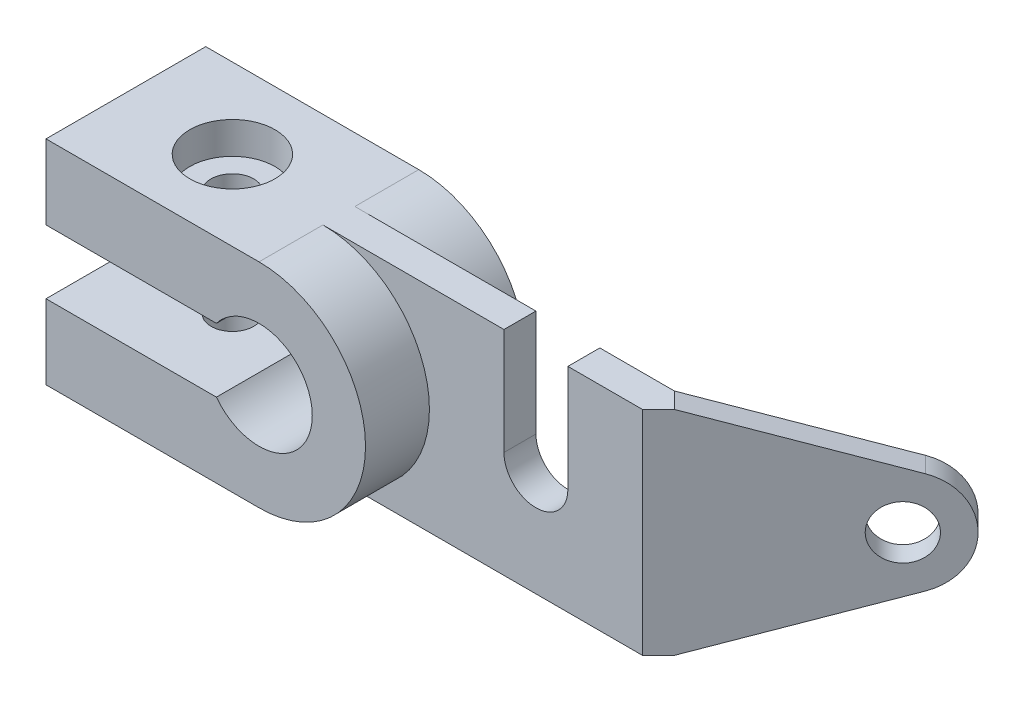
ISO-10303-21;
HEADER;
FILE_DESCRIPTION(('STEP AP214'),'2;1');
FILE_NAME('part.step','',(''),(''),'','','');
FILE_SCHEMA(('AUTOMOTIVE_DESIGN { 1 0 10303 214 1 1 1 1 }'));
ENDSEC;
DATA;
#1=APPLICATION_CONTEXT('core data for automotive mechanical design processes');
#2=APPLICATION_PROTOCOL_DEFINITION('international standard','automotive_design',2000,#1);
#3=PRODUCT_CONTEXT('',#1,'mechanical');
#4=PRODUCT('Part','Part','',(#3));
#5=PRODUCT_RELATED_PRODUCT_CATEGORY('part','',(#4));
#6=PRODUCT_DEFINITION_FORMATION('','',#4);
#7=PRODUCT_DEFINITION_CONTEXT('part definition',#1,'design');
#8=PRODUCT_DEFINITION('design','',#6,#7);
#9=PRODUCT_DEFINITION_SHAPE('','',#8);
#10=(LENGTH_UNIT() NAMED_UNIT(*) SI_UNIT(.MILLI.,.METRE.));
#11=(NAMED_UNIT(*) PLANE_ANGLE_UNIT() SI_UNIT($,.RADIAN.));
#12=(NAMED_UNIT(*) SI_UNIT($,.STERADIAN.) SOLID_ANGLE_UNIT());
#13=UNCERTAINTY_MEASURE_WITH_UNIT(LENGTH_MEASURE(1.E-05),#10,'distance_accuracy_value','');
#14=(GEOMETRIC_REPRESENTATION_CONTEXT(3) GLOBAL_UNCERTAINTY_ASSIGNED_CONTEXT((#13)) GLOBAL_UNIT_ASSIGNED_CONTEXT((#10,
#11,#12)) REPRESENTATION_CONTEXT('',''));
#15=CARTESIAN_POINT('',(0.,0.,0.));
#16=DIRECTION('',(0.,0.,1.));
#17=DIRECTION('',(1.,0.,0.));
#18=AXIS2_PLACEMENT_3D('',#15,#16,#17);
#19=CARTESIAN_POINT('',(90.,30.,4.5));
#20=DIRECTION('',(-0.707106781186549,0.,-0.707106781186546));
#21=DIRECTION('',(-0.707106781186546,0.,0.707106781186549));
#22=AXIS2_PLACEMENT_3D('',#19,#20,#21);
#23=PLANE('',#22);
#24=CARTESIAN_POINT('',(126.673358543988,0.,-32.173358543988));
#25=DIRECTION('',(-0.707106781186549,0.,-0.707106781186546));
#26=DIRECTION('',(-0.707106781186546,0.,0.707106781186549));
#27=AXIS2_PLACEMENT_3D('',#24,#25,#26);
#28=CIRCLE('',#27,7.50000000000002);
#29=CARTESIAN_POINT('',(121.370057685089,0.,-26.8700576850888));
#30=VERTEX_POINT('',#29);
#31=EDGE_CURVE('E220',#30,#30,#28,.T.);
#32=ORIENTED_EDGE('',*,*,#31,.T.);
#33=EDGE_LOOP('',(#32));
#34=FACE_BOUND('',#33,.T.);
#35=DIRECTION('',(0.674665588129938,0.299420587780075,-0.674665588129941));
#36=VECTOR('',#35,1.);
#37=CARTESIAN_POINT('',(102.523963114911,-26.4389175993817,-8.02396311491096));
#38=LINE('',#37,#36);
#39=CARTESIAN_POINT('',(94.5,-30.,0.));
#40=VERTEX_POINT('',#39);
#41=CARTESIAN_POINT('',(129.84919346468,-14.3118183719967,-35.3491934646803));
#42=VERTEX_POINT('',#41);
#43=EDGE_CURVE('E197',#40,#42,#38,.T.);
#44=ORIENTED_EDGE('',*,*,#43,.T.);
#45=CARTESIAN_POINT('',(126.673358543988,0.,-32.173358543988));
#46=DIRECTION('',(-0.707106781186549,0.,-0.707106781186546));
#47=DIRECTION('',(-0.707106781186546,0.,0.707106781186549));
#48=AXIS2_PLACEMENT_3D('',#45,#46,#47);
#49=CIRCLE('',#48,15.);
#50=CARTESIAN_POINT('',(129.84919346468,14.3118183719967,-35.3491934646803));
#51=VERTEX_POINT('',#50);
#52=EDGE_CURVE('E358',#51,#42,#49,.T.);
#53=ORIENTED_EDGE('',*,*,#52,.F.);
#54=DIRECTION('',(-0.674665588129938,0.299420587780076,0.674665588129941));
#55=VECTOR('',#54,1.);
#56=CARTESIAN_POINT('',(90.4034370977395,31.8180789025757,4.09656290226045));
#57=LINE('',#56,#55);
#58=CARTESIAN_POINT('',(94.5,30.,0.));
#59=VERTEX_POINT('',#58);
#60=EDGE_CURVE('E352',#51,#59,#57,.T.);
#61=ORIENTED_EDGE('',*,*,#60,.T.);
#62=DIRECTION('',(0.707106781186546,0.,-0.707106781186549));
#63=VECTOR('',#62,1.);
#64=CARTESIAN_POINT('',(90.,30.,4.5));
#65=LINE('',#64,#63);
#66=CARTESIAN_POINT('',(90.,30.,4.5));
#67=VERTEX_POINT('',#66);
#68=EDGE_CURVE('E353',#67,#59,#65,.T.);
#69=ORIENTED_EDGE('',*,*,#68,.F.);
#70=DIRECTION('',(0.,-1.,0.));
#71=VECTOR('',#70,1.);
#72=CARTESIAN_POINT('',(90.,30.,4.5));
#73=LINE('',#72,#71);
#74=CARTESIAN_POINT('',(90.,-30.,4.5));
#75=VERTEX_POINT('',#74);
#76=EDGE_CURVE('E222',#67,#75,#73,.T.);
#77=ORIENTED_EDGE('',*,*,#76,.T.);
#78=DIRECTION('',(0.707106781186546,0.,-0.707106781186549));
#79=VECTOR('',#78,1.);
#80=CARTESIAN_POINT('',(90.,-30.,4.5));
#81=LINE('',#80,#79);
#82=EDGE_CURVE('E218',#75,#40,#81,.T.);
#83=ORIENTED_EDGE('',*,*,#82,.T.);
#84=EDGE_LOOP('',(#44,#53,#61,#69,#77,#83));
#85=FACE_BOUND('',#84,.T.);
#86=ADVANCED_FACE('F69',(#34,#85),#23,.F.);
#87=CARTESIAN_POINT('',(132.779960261786,30.,-47.2799602617859));
#88=DIRECTION('',(0.707106781186544,0.,0.707106781186551));
#89=DIRECTION('',(0.707106781186551,0.,-0.707106781186544));
#90=AXIS2_PLACEMENT_3D('',#87,#88,#89);
#91=PLANE('',#90);
#92=CARTESIAN_POINT('',(122.173358543988,0.,-36.6733585439877));
#93=DIRECTION('',(0.707106781186544,0.,0.707106781186551));
#94=DIRECTION('',(0.707106781186551,0.,-0.707106781186544));
#95=AXIS2_PLACEMENT_3D('',#92,#93,#94);
#96=CIRCLE('',#95,7.50000000000002);
#97=CARTESIAN_POINT('',(127.476659402887,0.,-41.9766594028868));
#98=VERTEX_POINT('',#97);
#99=EDGE_CURVE('E71',#98,#98,#96,.T.);
#100=ORIENTED_EDGE('',*,*,#99,.T.);
#101=EDGE_LOOP('',(#100));
#102=FACE_BOUND('',#101,.T.);
#103=CARTESIAN_POINT('',(122.173358543988,0.,-36.6733585439877));
#104=DIRECTION('',(0.707106781186544,0.,0.707106781186551));
#105=DIRECTION('',(0.707106781186551,0.,-0.707106781186544));
#106=AXIS2_PLACEMENT_3D('',#103,#104,#105);
#107=CIRCLE('',#106,15.);
#108=CARTESIAN_POINT('',(125.34919346468,-14.3118183719967,-39.84919346468));
#109=VERTEX_POINT('',#108);
#110=CARTESIAN_POINT('',(125.34919346468,14.3118183719967,-39.84919346468));
#111=VERTEX_POINT('',#110);
#112=EDGE_CURVE('E12',#109,#111,#107,.T.);
#113=ORIENTED_EDGE('',*,*,#112,.F.);
#114=DIRECTION('',(-0.674665588129943,-0.299420587780075,0.674665588129936));
#115=VECTOR('',#114,1.);
#116=CARTESIAN_POINT('',(141.065147832418,-7.33698465125482,-55.5651478324177));
#117=LINE('',#116,#115);
#118=CARTESIAN_POINT('',(90.,-30.,-4.5));
#119=VERTEX_POINT('',#118);
#120=EDGE_CURVE('E209',#109,#119,#117,.T.);
#121=ORIENTED_EDGE('',*,*,#120,.T.);
#122=DIRECTION('',(0.,-1.,0.));
#123=VECTOR('',#122,1.);
#124=CARTESIAN_POINT('',(90.,30.,-4.5));
#125=LINE('',#124,#123);
#126=CARTESIAN_POINT('',(90.,30.,-4.5));
#127=VERTEX_POINT('',#126);
#128=EDGE_CURVE('E231',#127,#119,#125,.T.);
#129=ORIENTED_EDGE('',*,*,#128,.F.);
#130=DIRECTION('',(0.674665588129943,-0.299420587780076,-0.674665588129936));
#131=VECTOR('',#130,1.);
#132=CARTESIAN_POINT('',(128.944621815247,12.7161459544488,-43.4446218152463));
#133=LINE('',#132,#131);
#134=EDGE_CURVE('E77',#127,#111,#133,.T.);
#135=ORIENTED_EDGE('',*,*,#134,.T.);
#136=EDGE_LOOP('',(#113,#121,#129,#135));
#137=FACE_BOUND('',#136,.T.);
#138=ADVANCED_FACE('F345',(#102,#137),#91,.F.);
#139=CARTESIAN_POINT('',(0.,30.,22.5));
#140=DIRECTION('',(0.,-1.,0.));
#141=DIRECTION('',(1.,0.,0.));
#142=AXIS2_PLACEMENT_3D('',#139,#140,#141);
#143=PLANE('',#142);
#144=CARTESIAN_POINT('',(-30.,30.,0.));
#145=DIRECTION('',(0.,1.,0.));
#146=DIRECTION('',(-1.,0.,0.));
#147=AXIS2_PLACEMENT_3D('',#144,#145,#146);
#148=CIRCLE('',#147,12.);
#149=CARTESIAN_POINT('',(-42.,30.,0.));
#150=VERTEX_POINT('',#149);
#151=EDGE_CURVE('E263',#150,#150,#148,.T.);
#152=ORIENTED_EDGE('',*,*,#151,.F.);
#153=EDGE_LOOP('',(#152));
#154=FACE_BOUND('',#153,.T.);
#155=DIRECTION('',(0.,0.,-1.));
#156=VECTOR('',#155,1.);
#157=CARTESIAN_POINT('',(51.,30.,25.5));
#158=LINE('',#157,#156);
#159=CARTESIAN_POINT('',(51.,30.,4.5));
#160=VERTEX_POINT('',#159);
#161=CARTESIAN_POINT('',(51.,30.,-4.5));
#162=VERTEX_POINT('',#161);
#163=EDGE_CURVE('E362',#160,#162,#158,.T.);
#164=ORIENTED_EDGE('',*,*,#163,.T.);
#165=DIRECTION('',(-1.,0.,0.));
#166=VECTOR('',#165,1.);
#167=CARTESIAN_POINT('',(0.,30.,-4.5));
#168=LINE('',#167,#166);
#169=CARTESIAN_POINT('',(0.,30.,-4.49999999999999));
#170=VERTEX_POINT('',#169);
#171=EDGE_CURVE('E382',#162,#170,#168,.T.);
#172=ORIENTED_EDGE('',*,*,#171,.T.);
#173=DIRECTION('',(0.,0.,-1.));
#174=VECTOR('',#173,1.);
#175=CARTESIAN_POINT('',(0.,30.,22.5));
#176=LINE('',#175,#174);
#177=CARTESIAN_POINT('',(0.,30.,-22.5));
#178=VERTEX_POINT('',#177);
#179=EDGE_CURVE('E316',#170,#178,#176,.T.);
#180=ORIENTED_EDGE('',*,*,#179,.T.);
#181=DIRECTION('',(-1.,0.,0.));
#182=VECTOR('',#181,1.);
#183=CARTESIAN_POINT('',(0.,30.,-22.5));
#184=LINE('',#183,#182);
#185=CARTESIAN_POINT('',(-60.,30.,-22.5));
#186=VERTEX_POINT('',#185);
#187=EDGE_CURVE('E293',#178,#186,#184,.T.);
#188=ORIENTED_EDGE('',*,*,#187,.T.);
#189=DIRECTION('',(0.,0.,-1.));
#190=VECTOR('',#189,1.);
#191=CARTESIAN_POINT('',(-60.,30.,22.5));
#192=LINE('',#191,#190);
#193=CARTESIAN_POINT('',(-60.,30.,22.5));
#194=VERTEX_POINT('',#193);
#195=EDGE_CURVE('E320',#194,#186,#192,.T.);
#196=ORIENTED_EDGE('',*,*,#195,.F.);
#197=DIRECTION('',(-1.,0.,0.));
#198=VECTOR('',#197,1.);
#199=CARTESIAN_POINT('',(0.,30.,22.5));
#200=LINE('',#199,#198);
#201=CARTESIAN_POINT('',(0.,30.,22.5));
#202=VERTEX_POINT('',#201);
#203=EDGE_CURVE('E269',#202,#194,#200,.T.);
#204=ORIENTED_EDGE('',*,*,#203,.F.);
#205=CARTESIAN_POINT('',(0.,30.,4.5));
#206=VERTEX_POINT('',#205);
#207=EDGE_CURVE('E318',#202,#206,#176,.T.);
#208=ORIENTED_EDGE('',*,*,#207,.T.);
#209=DIRECTION('',(1.,0.,0.));
#210=VECTOR('',#209,1.);
#211=CARTESIAN_POINT('',(0.,30.,4.5));
#212=LINE('',#211,#210);
#213=EDGE_CURVE('E377',#206,#160,#212,.T.);
#214=ORIENTED_EDGE('',*,*,#213,.T.);
#215=EDGE_LOOP('',(#164,#172,#180,#188,#196,#204,#208,#214));
#216=FACE_BOUND('',#215,.T.);
#217=ADVANCED_FACE('F381',(#154,#216),#143,.F.);
#218=CARTESIAN_POINT('',(0.,0.,22.5));
#219=DIRECTION('',(0.,0.,-1.));
#220=DIRECTION('',(-1.,0.,0.));
#221=AXIS2_PLACEMENT_3D('',#218,#219,#220);
#222=CYLINDRICAL_SURFACE('',#221,30.);
#223=CARTESIAN_POINT('',(0.,0.,4.5));
#224=DIRECTION('',(0.,0.,-1.));
#225=DIRECTION('',(-1.,0.,0.));
#226=AXIS2_PLACEMENT_3D('',#223,#224,#225);
#227=CIRCLE('',#226,30.);
#228=CARTESIAN_POINT('',(0.,-30.,4.5));
#229=VERTEX_POINT('',#228);
#230=EDGE_CURVE('E241',#206,#229,#227,.T.);
#231=ORIENTED_EDGE('',*,*,#230,.F.);
#232=ORIENTED_EDGE('',*,*,#207,.F.);
#233=CARTESIAN_POINT('',(0.,0.,22.5));
#234=DIRECTION('',(0.,0.,1.));
#235=DIRECTION('',(1.,0.,0.));
#236=AXIS2_PLACEMENT_3D('',#233,#234,#235);
#237=CIRCLE('',#236,30.);
#238=CARTESIAN_POINT('',(0.,-30.,22.5));
#239=VERTEX_POINT('',#238);
#240=EDGE_CURVE('E270',#239,#202,#237,.T.);
#241=ORIENTED_EDGE('',*,*,#240,.F.);
#242=DIRECTION('',(0.,0.,-1.));
#243=VECTOR('',#242,1.);
#244=CARTESIAN_POINT('',(0.,-30.,22.5));
#245=LINE('',#244,#243);
#246=EDGE_CURVE('E321',#239,#229,#245,.T.);
#247=ORIENTED_EDGE('',*,*,#246,.T.);
#248=EDGE_LOOP('',(#231,#232,#241,#247));
#249=FACE_BOUND('',#248,.T.);
#250=ADVANCED_FACE('F426',(#249),#222,.T.);
#251=CARTESIAN_POINT('',(0.,0.,-4.5));
#252=DIRECTION('',(0.,0.,1.));
#253=DIRECTION('',(1.,0.,0.));
#254=AXIS2_PLACEMENT_3D('',#251,#252,#253);
#255=CIRCLE('',#254,30.);
#256=CARTESIAN_POINT('',(0.,-30.,-4.5));
#257=VERTEX_POINT('',#256);
#258=EDGE_CURVE('E238',#257,#170,#255,.T.);
#259=ORIENTED_EDGE('',*,*,#258,.F.);
#260=CARTESIAN_POINT('',(0.,-30.,-22.5));
#261=VERTEX_POINT('',#260);
#262=EDGE_CURVE('E324',#257,#261,#245,.T.);
#263=ORIENTED_EDGE('',*,*,#262,.T.);
#264=CARTESIAN_POINT('',(0.,0.,-22.5));
#265=DIRECTION('',(0.,0.,1.));
#266=DIRECTION('',(1.,0.,0.));
#267=AXIS2_PLACEMENT_3D('',#264,#265,#266);
#268=CIRCLE('',#267,30.);
#269=EDGE_CURVE('E288',#261,#178,#268,.T.);
#270=ORIENTED_EDGE('',*,*,#269,.T.);
#271=ORIENTED_EDGE('',*,*,#179,.F.);
#272=EDGE_LOOP('',(#259,#263,#270,#271));
#273=FACE_BOUND('',#272,.T.);
#274=ADVANCED_FACE('F393',(#273),#222,.T.);
#275=CARTESIAN_POINT('',(0.,0.,22.5));
#276=DIRECTION('',(0.,0.,-1.));
#277=DIRECTION('',(-1.,0.,0.));
#278=AXIS2_PLACEMENT_3D('',#275,#276,#277);
#279=CYLINDRICAL_SURFACE('',#278,15.);
#280=DIRECTION('',(0.,0.,-1.));
#281=VECTOR('',#280,1.);
#282=CARTESIAN_POINT('',(-12.,9.,22.5));
#283=LINE('',#282,#281);
#284=CARTESIAN_POINT('',(-12.,9.,22.5));
#285=VERTEX_POINT('',#284);
#286=CARTESIAN_POINT('',(-12.,9.,-22.5));
#287=VERTEX_POINT('',#286);
#288=EDGE_CURVE('E315',#285,#287,#283,.T.);
#289=ORIENTED_EDGE('',*,*,#288,.T.);
#290=CARTESIAN_POINT('',(0.,0.,-22.5));
#291=DIRECTION('',(0.,0.,1.));
#292=DIRECTION('',(1.,0.,0.));
#293=AXIS2_PLACEMENT_3D('',#290,#291,#292);
#294=CIRCLE('',#293,15.);
#295=CARTESIAN_POINT('',(-12.,-9.,-22.5));
#296=VERTEX_POINT('',#295);
#297=EDGE_CURVE('E297',#296,#287,#294,.T.);
#298=ORIENTED_EDGE('',*,*,#297,.F.);
#299=DIRECTION('',(0.,0.,-1.));
#300=VECTOR('',#299,1.);
#301=CARTESIAN_POINT('',(-12.,-9.,22.5));
#302=LINE('',#301,#300);
#303=CARTESIAN_POINT('',(-12.,-9.,22.5));
#304=VERTEX_POINT('',#303);
#305=EDGE_CURVE('E309',#304,#296,#302,.T.);
#306=ORIENTED_EDGE('',*,*,#305,.F.);
#307=CARTESIAN_POINT('',(0.,0.,22.5));
#308=DIRECTION('',(0.,0.,1.));
#309=DIRECTION('',(1.,0.,0.));
#310=AXIS2_PLACEMENT_3D('',#307,#308,#309);
#311=CIRCLE('',#310,15.);
#312=EDGE_CURVE('E279',#304,#285,#311,.T.);
#313=ORIENTED_EDGE('',*,*,#312,.T.);
#314=EDGE_LOOP('',(#289,#298,#306,#313));
#315=FACE_BOUND('',#314,.T.);
#316=ADVANCED_FACE('F415',(#315),#279,.F.);
#317=CARTESIAN_POINT('',(0.,-30.,22.5));
#318=DIRECTION('',(0.,-1.,0.));
#319=DIRECTION('',(1.,0.,0.));
#320=AXIS2_PLACEMENT_3D('',#317,#318,#319);
#321=PLANE('',#320);
#322=DIRECTION('',(-0.707106781186544,0.,-0.707106781186551));
#323=VECTOR('',#322,1.);
#324=CARTESIAN_POINT('',(111.213203435596,-30.,16.7132034355965));
#325=LINE('',#324,#323);
#326=EDGE_CURVE('E205',#40,#119,#325,.T.);
#327=ORIENTED_EDGE('',*,*,#326,.F.);
#328=ORIENTED_EDGE('',*,*,#82,.F.);
#329=DIRECTION('',(1.,0.,0.));
#330=VECTOR('',#329,1.);
#331=CARTESIAN_POINT('',(0.,-30.,4.5));
#332=LINE('',#331,#330);
#333=EDGE_CURVE('E224',#229,#75,#332,.T.);
#334=ORIENTED_EDGE('',*,*,#333,.F.);
#335=ORIENTED_EDGE('',*,*,#246,.F.);
#336=DIRECTION('',(-1.,0.,0.));
#337=VECTOR('',#336,1.);
#338=CARTESIAN_POINT('',(0.,-30.,22.5));
#339=LINE('',#338,#337);
#340=CARTESIAN_POINT('',(-60.,-30.,22.5));
#341=VERTEX_POINT('',#340);
#342=EDGE_CURVE('E265',#239,#341,#339,.T.);
#343=ORIENTED_EDGE('',*,*,#342,.T.);
#344=DIRECTION('',(0.,0.,-1.));
#345=VECTOR('',#344,1.);
#346=CARTESIAN_POINT('',(-60.,-30.,22.5));
#347=LINE('',#346,#345);
#348=CARTESIAN_POINT('',(-60.,-30.,-22.5));
#349=VERTEX_POINT('',#348);
#350=EDGE_CURVE('E281',#341,#349,#347,.T.);
#351=ORIENTED_EDGE('',*,*,#350,.T.);
#352=DIRECTION('',(-1.,0.,0.));
#353=VECTOR('',#352,1.);
#354=CARTESIAN_POINT('',(0.,-30.,-22.5));
#355=LINE('',#354,#353);
#356=EDGE_CURVE('E258',#261,#349,#355,.T.);
#357=ORIENTED_EDGE('',*,*,#356,.F.);
#358=ORIENTED_EDGE('',*,*,#262,.F.);
#359=DIRECTION('',(-1.,0.,0.));
#360=VECTOR('',#359,1.);
#361=CARTESIAN_POINT('',(0.,-30.,-4.5));
#362=LINE('',#361,#360);
#363=EDGE_CURVE('E217',#119,#257,#362,.T.);
#364=ORIENTED_EDGE('',*,*,#363,.F.);
#365=EDGE_LOOP('',(#327,#328,#334,#335,#343,#351,#357,#358,#364));
#366=FACE_BOUND('',#365,.T.);
#367=CARTESIAN_POINT('',(-30.,-30.,0.));
#368=DIRECTION('',(0.,1.,0.));
#369=DIRECTION('',(-1.,0.,0.));
#370=AXIS2_PLACEMENT_3D('',#367,#368,#369);
#371=CIRCLE('',#370,12.);
#372=CARTESIAN_POINT('',(-42.,-30.,0.));
#373=VERTEX_POINT('',#372);
#374=EDGE_CURVE('E252',#373,#373,#371,.T.);
#375=ORIENTED_EDGE('',*,*,#374,.T.);
#376=EDGE_LOOP('',(#375));
#377=FACE_BOUND('',#376,.T.);
#378=ADVANCED_FACE('F70',(#366,#377),#321,.T.);
#379=ORIENTED_EDGE('',*,*,#68,.T.);
#380=DIRECTION('',(-0.707106781186544,0.,-0.707106781186551));
#381=VECTOR('',#380,1.);
#382=CARTESIAN_POINT('',(111.213203435596,30.,16.7132034355965));
#383=LINE('',#382,#381);
#384=EDGE_CURVE('E348',#59,#127,#383,.T.);
#385=ORIENTED_EDGE('',*,*,#384,.T.);
#386=CARTESIAN_POINT('',(69.,30.,-4.5));
#387=VERTEX_POINT('',#386);
#388=EDGE_CURVE('E236',#127,#387,#168,.T.);
#389=ORIENTED_EDGE('',*,*,#388,.T.);
#390=DIRECTION('',(0.,0.,-1.));
#391=VECTOR('',#390,1.);
#392=CARTESIAN_POINT('',(69.,30.,25.5));
#393=LINE('',#392,#391);
#394=CARTESIAN_POINT('',(69.,30.,4.5));
#395=VERTEX_POINT('',#394);
#396=EDGE_CURVE('E365',#395,#387,#393,.T.);
#397=ORIENTED_EDGE('',*,*,#396,.F.);
#398=EDGE_CURVE('E227',#395,#67,#212,.T.);
#399=ORIENTED_EDGE('',*,*,#398,.T.);
#400=EDGE_LOOP('',(#379,#385,#389,#397,#399));
#401=FACE_BOUND('',#400,.T.);
#402=ADVANCED_FACE('F351',(#401),#143,.F.);
#403=CARTESIAN_POINT('',(-60.,0.,22.5));
#404=DIRECTION('',(-1.,0.,0.));
#405=DIRECTION('',(0.,0.,1.));
#406=AXIS2_PLACEMENT_3D('',#403,#404,#405);
#407=PLANE('',#406);
#408=DIRECTION('',(0.,1.,0.));
#409=VECTOR('',#408,1.);
#410=CARTESIAN_POINT('',(-60.,0.,-22.5));
#411=LINE('',#410,#409);
#412=CARTESIAN_POINT('',(-60.,9.,-22.5));
#413=VERTEX_POINT('',#412);
#414=EDGE_CURVE('E295',#413,#186,#411,.T.);
#415=ORIENTED_EDGE('',*,*,#414,.F.);
#416=DIRECTION('',(0.,0.,-1.));
#417=VECTOR('',#416,1.);
#418=CARTESIAN_POINT('',(-60.,9.,22.5));
#419=LINE('',#418,#417);
#420=CARTESIAN_POINT('',(-60.,9.,22.5));
#421=VERTEX_POINT('',#420);
#422=EDGE_CURVE('E314',#421,#413,#419,.T.);
#423=ORIENTED_EDGE('',*,*,#422,.F.);
#424=DIRECTION('',(0.,1.,0.));
#425=VECTOR('',#424,1.);
#426=CARTESIAN_POINT('',(-60.,0.,22.5));
#427=LINE('',#426,#425);
#428=EDGE_CURVE('E275',#421,#194,#427,.T.);
#429=ORIENTED_EDGE('',*,*,#428,.T.);
#430=ORIENTED_EDGE('',*,*,#195,.T.);
#431=EDGE_LOOP('',(#415,#423,#429,#430));
#432=FACE_BOUND('',#431,.T.);
#433=ADVANCED_FACE('F405',(#432),#407,.T.);
#434=CARTESIAN_POINT('',(0.,9.,22.5));
#435=DIRECTION('',(0.,-1.,0.));
#436=DIRECTION('',(1.,0.,0.));
#437=AXIS2_PLACEMENT_3D('',#434,#435,#436);
#438=PLANE('',#437);
#439=CARTESIAN_POINT('',(-30.,9.,0.));
#440=DIRECTION('',(0.,1.,0.));
#441=DIRECTION('',(-1.,0.,0.));
#442=AXIS2_PLACEMENT_3D('',#439,#440,#441);
#443=CIRCLE('',#442,6.);
#444=CARTESIAN_POINT('',(-36.,9.,0.));
#445=VERTEX_POINT('',#444);
#446=EDGE_CURVE('E249',#445,#445,#443,.T.);
#447=ORIENTED_EDGE('',*,*,#446,.T.);
#448=EDGE_LOOP('',(#447));
#449=FACE_BOUND('',#448,.T.);
#450=DIRECTION('',(-1.,0.,0.));
#451=VECTOR('',#450,1.);
#452=CARTESIAN_POINT('',(0.,9.,-22.5));
#453=LINE('',#452,#451);
#454=EDGE_CURVE('E300',#287,#413,#453,.T.);
#455=ORIENTED_EDGE('',*,*,#454,.F.);
#456=ORIENTED_EDGE('',*,*,#288,.F.);
#457=DIRECTION('',(-1.,0.,0.));
#458=VECTOR('',#457,1.);
#459=CARTESIAN_POINT('',(0.,9.,22.5));
#460=LINE('',#459,#458);
#461=EDGE_CURVE('E273',#285,#421,#460,.T.);
#462=ORIENTED_EDGE('',*,*,#461,.T.);
#463=ORIENTED_EDGE('',*,*,#422,.T.);
#464=EDGE_LOOP('',(#455,#456,#462,#463));
#465=FACE_BOUND('',#464,.T.);
#466=ADVANCED_FACE('F413',(#449,#465),#438,.T.);
#467=CARTESIAN_POINT('',(0.,-8.99999999999999,22.5));
#468=DIRECTION('',(0.,-1.,0.));
#469=DIRECTION('',(1.,0.,0.));
#470=AXIS2_PLACEMENT_3D('',#467,#468,#469);
#471=PLANE('',#470);
#472=CARTESIAN_POINT('',(-30.,-9.,0.));
#473=DIRECTION('',(0.,1.,0.));
#474=DIRECTION('',(-1.,0.,0.));
#475=AXIS2_PLACEMENT_3D('',#472,#473,#474);
#476=CIRCLE('',#475,6.);
#477=CARTESIAN_POINT('',(-24.,-9.,0.));
#478=VERTEX_POINT('',#477);
#479=EDGE_CURVE('E243',#478,#478,#476,.T.);
#480=ORIENTED_EDGE('',*,*,#479,.F.);
#481=EDGE_LOOP('',(#480));
#482=FACE_BOUND('',#481,.T.);
#483=DIRECTION('',(-1.,0.,0.));
#484=VECTOR('',#483,1.);
#485=CARTESIAN_POINT('',(0.,-8.99999999999999,-22.5));
#486=LINE('',#485,#484);
#487=CARTESIAN_POINT('',(-60.,-9.,-22.5));
#488=VERTEX_POINT('',#487);
#489=EDGE_CURVE('E305',#296,#488,#486,.T.);
#490=ORIENTED_EDGE('',*,*,#489,.T.);
#491=DIRECTION('',(0.,0.,-1.));
#492=VECTOR('',#491,1.);
#493=CARTESIAN_POINT('',(-60.,-9.,22.5));
#494=LINE('',#493,#492);
#495=CARTESIAN_POINT('',(-60.,-9.,22.5));
#496=VERTEX_POINT('',#495);
#497=EDGE_CURVE('E308',#496,#488,#494,.T.);
#498=ORIENTED_EDGE('',*,*,#497,.F.);
#499=DIRECTION('',(-1.,0.,0.));
#500=VECTOR('',#499,1.);
#501=CARTESIAN_POINT('',(0.,-8.99999999999999,22.5));
#502=LINE('',#501,#500);
#503=EDGE_CURVE('E278',#304,#496,#502,.T.);
#504=ORIENTED_EDGE('',*,*,#503,.F.);
#505=ORIENTED_EDGE('',*,*,#305,.T.);
#506=EDGE_LOOP('',(#490,#498,#504,#505));
#507=FACE_BOUND('',#506,.T.);
#508=ADVANCED_FACE('F417',(#482,#507),#471,.F.);
#509=CARTESIAN_POINT('',(-60.,0.,22.5));
#510=DIRECTION('',(-1.,0.,0.));
#511=DIRECTION('',(0.,0.,1.));
#512=AXIS2_PLACEMENT_3D('',#509,#510,#511);
#513=PLANE('',#512);
#514=DIRECTION('',(0.,1.,0.));
#515=VECTOR('',#514,1.);
#516=CARTESIAN_POINT('',(-60.,0.,-22.5));
#517=LINE('',#516,#515);
#518=EDGE_CURVE('E268',#349,#488,#517,.T.);
#519=ORIENTED_EDGE('',*,*,#518,.F.);
#520=ORIENTED_EDGE('',*,*,#350,.F.);
#521=DIRECTION('',(0.,1.,0.));
#522=VECTOR('',#521,1.);
#523=CARTESIAN_POINT('',(-60.,0.,22.5));
#524=LINE('',#523,#522);
#525=EDGE_CURVE('E284',#341,#496,#524,.T.);
#526=ORIENTED_EDGE('',*,*,#525,.T.);
#527=ORIENTED_EDGE('',*,*,#497,.T.);
#528=EDGE_LOOP('',(#519,#520,#526,#527));
#529=FACE_BOUND('',#528,.T.);
#530=ADVANCED_FACE('F421',(#529),#513,.T.);
#531=CARTESIAN_POINT('',(0.,0.,22.5));
#532=DIRECTION('',(0.,0.,1.));
#533=DIRECTION('',(1.,0.,0.));
#534=AXIS2_PLACEMENT_3D('',#531,#532,#533);
#535=PLANE('',#534);
#536=ORIENTED_EDGE('',*,*,#342,.F.);
#537=ORIENTED_EDGE('',*,*,#240,.T.);
#538=ORIENTED_EDGE('',*,*,#203,.T.);
#539=ORIENTED_EDGE('',*,*,#428,.F.);
#540=ORIENTED_EDGE('',*,*,#461,.F.);
#541=ORIENTED_EDGE('',*,*,#312,.F.);
#542=ORIENTED_EDGE('',*,*,#503,.T.);
#543=ORIENTED_EDGE('',*,*,#525,.F.);
#544=EDGE_LOOP('',(#536,#537,#538,#539,#540,#541,#542,#543));
#545=FACE_BOUND('',#544,.T.);
#546=ADVANCED_FACE('F407',(#545),#535,.T.);
#547=CARTESIAN_POINT('',(0.,0.,-22.5));
#548=DIRECTION('',(0.,0.,1.));
#549=DIRECTION('',(1.,0.,0.));
#550=AXIS2_PLACEMENT_3D('',#547,#548,#549);
#551=PLANE('',#550);
#552=ORIENTED_EDGE('',*,*,#356,.T.);
#553=ORIENTED_EDGE('',*,*,#518,.T.);
#554=ORIENTED_EDGE('',*,*,#489,.F.);
#555=ORIENTED_EDGE('',*,*,#297,.T.);
#556=ORIENTED_EDGE('',*,*,#454,.T.);
#557=ORIENTED_EDGE('',*,*,#414,.T.);
#558=ORIENTED_EDGE('',*,*,#187,.F.);
#559=ORIENTED_EDGE('',*,*,#269,.F.);
#560=EDGE_LOOP('',(#552,#553,#554,#555,#556,#557,#558,#559));
#561=FACE_BOUND('',#560,.T.);
#562=ADVANCED_FACE('F396',(#561),#551,.F.);
#563=CARTESIAN_POINT('',(-30.,21.,0.));
#564=DIRECTION('',(0.,1.,0.));
#565=DIRECTION('',(-1.,0.,0.));
#566=AXIS2_PLACEMENT_3D('',#563,#564,#565);
#567=CYLINDRICAL_SURFACE('',#566,12.);
#568=CARTESIAN_POINT('',(-30.,21.,0.));
#569=DIRECTION('',(0.,1.,0.));
#570=DIRECTION('',(-1.,0.,0.));
#571=AXIS2_PLACEMENT_3D('',#568,#569,#570);
#572=CIRCLE('',#571,12.);
#573=CARTESIAN_POINT('',(-42.,21.,0.));
#574=VERTEX_POINT('',#573);
#575=EDGE_CURVE('E260',#574,#574,#572,.T.);
#576=ORIENTED_EDGE('',*,*,#575,.F.);
#577=EDGE_LOOP('',(#576));
#578=FACE_BOUND('',#577,.T.);
#579=ORIENTED_EDGE('',*,*,#151,.T.);
#580=EDGE_LOOP('',(#579));
#581=FACE_BOUND('',#580,.T.);
#582=ADVANCED_FACE('F486',(#578,#581),#567,.F.);
#583=CARTESIAN_POINT('',(-30.,21.,0.));
#584=DIRECTION('',(0.,1.,0.));
#585=DIRECTION('',(-1.,0.,0.));
#586=AXIS2_PLACEMENT_3D('',#583,#584,#585);
#587=PLANE('',#586);
#588=CARTESIAN_POINT('',(-30.,21.,0.));
#589=DIRECTION('',(0.,1.,0.));
#590=DIRECTION('',(-1.,0.,0.));
#591=AXIS2_PLACEMENT_3D('',#588,#589,#590);
#592=CIRCLE('',#591,6.);
#593=CARTESIAN_POINT('',(-36.,21.,0.));
#594=VERTEX_POINT('',#593);
#595=EDGE_CURVE('E257',#594,#594,#592,.T.);
#596=ORIENTED_EDGE('',*,*,#595,.F.);
#597=EDGE_LOOP('',(#596));
#598=FACE_BOUND('',#597,.T.);
#599=ORIENTED_EDGE('',*,*,#575,.T.);
#600=EDGE_LOOP('',(#599));
#601=FACE_BOUND('',#600,.T.);
#602=ADVANCED_FACE('F482',(#598,#601),#587,.T.);
#603=CARTESIAN_POINT('',(-30.,9.,0.));
#604=DIRECTION('',(0.,1.,0.));
#605=DIRECTION('',(-1.,0.,0.));
#606=AXIS2_PLACEMENT_3D('',#603,#604,#605);
#607=CYLINDRICAL_SURFACE('',#606,6.);
#608=CARTESIAN_POINT('',(-36.,21.,0.));
#609=CARTESIAN_POINT('',(-36.,20.875,0.));
#610=CARTESIAN_POINT('',(-36.,20.75,0.));
#611=CARTESIAN_POINT('',(-36.,20.5,0.));
#612=CARTESIAN_POINT('',(-36.,20.375,0.));
#613=CARTESIAN_POINT('',(-36.,20.125,0.));
#614=CARTESIAN_POINT('',(-36.,20.,0.));
#615=CARTESIAN_POINT('',(-36.,19.75,0.));
#616=CARTESIAN_POINT('',(-36.,19.625,0.));
#617=CARTESIAN_POINT('',(-36.,19.375,0.));
#618=CARTESIAN_POINT('',(-36.,19.25,0.));
#619=CARTESIAN_POINT('',(-36.,19.,0.));
#620=CARTESIAN_POINT('',(-36.,18.875,0.));
#621=CARTESIAN_POINT('',(-36.,18.625,0.));
#622=CARTESIAN_POINT('',(-36.,18.5,0.));
#623=CARTESIAN_POINT('',(-36.,18.25,0.));
#624=CARTESIAN_POINT('',(-36.,18.125,0.));
#625=CARTESIAN_POINT('',(-36.,17.875,0.));
#626=CARTESIAN_POINT('',(-36.,17.75,0.));
#627=CARTESIAN_POINT('',(-36.,17.5,0.));
#628=CARTESIAN_POINT('',(-36.,17.375,0.));
#629=CARTESIAN_POINT('',(-36.,17.125,0.));
#630=CARTESIAN_POINT('',(-36.,17.,0.));
#631=CARTESIAN_POINT('',(-36.,16.75,0.));
#632=CARTESIAN_POINT('',(-36.,16.625,0.));
#633=CARTESIAN_POINT('',(-36.,16.375,0.));
#634=CARTESIAN_POINT('',(-36.,16.25,0.));
#635=CARTESIAN_POINT('',(-36.,16.,0.));
#636=CARTESIAN_POINT('',(-36.,15.875,0.));
#637=CARTESIAN_POINT('',(-36.,15.625,0.));
#638=CARTESIAN_POINT('',(-36.,15.5,0.));
#639=CARTESIAN_POINT('',(-36.,15.25,0.));
#640=CARTESIAN_POINT('',(-36.,15.125,0.));
#641=CARTESIAN_POINT('',(-36.,14.875,0.));
#642=CARTESIAN_POINT('',(-36.,14.75,0.));
#643=CARTESIAN_POINT('',(-36.,14.5,0.));
#644=CARTESIAN_POINT('',(-36.,14.375,0.));
#645=CARTESIAN_POINT('',(-36.,14.125,0.));
#646=CARTESIAN_POINT('',(-36.,14.,0.));
#647=CARTESIAN_POINT('',(-36.,13.75,0.));
#648=CARTESIAN_POINT('',(-36.,13.625,0.));
#649=CARTESIAN_POINT('',(-36.,13.375,0.));
#650=CARTESIAN_POINT('',(-36.,13.25,0.));
#651=CARTESIAN_POINT('',(-36.,13.,0.));
#652=CARTESIAN_POINT('',(-36.,12.875,0.));
#653=CARTESIAN_POINT('',(-36.,12.625,0.));
#654=CARTESIAN_POINT('',(-36.,12.5,0.));
#655=CARTESIAN_POINT('',(-36.,12.25,0.));
#656=CARTESIAN_POINT('',(-36.,12.125,0.));
#657=CARTESIAN_POINT('',(-36.,11.875,0.));
#658=CARTESIAN_POINT('',(-36.,11.75,0.));
#659=CARTESIAN_POINT('',(-36.,11.5,0.));
#660=CARTESIAN_POINT('',(-36.,11.375,0.));
#661=CARTESIAN_POINT('',(-36.,11.125,0.));
#662=CARTESIAN_POINT('',(-36.,11.,0.));
#663=CARTESIAN_POINT('',(-36.,10.75,0.));
#664=CARTESIAN_POINT('',(-36.,10.625,0.));
#665=CARTESIAN_POINT('',(-36.,10.375,0.));
#666=CARTESIAN_POINT('',(-36.,10.25,0.));
#667=CARTESIAN_POINT('',(-36.,10.,0.));
#668=CARTESIAN_POINT('',(-36.,9.875,0.));
#669=CARTESIAN_POINT('',(-36.,9.625,0.));
#670=CARTESIAN_POINT('',(-36.,9.5,0.));
#671=CARTESIAN_POINT('',(-36.,9.25,0.));
#672=CARTESIAN_POINT('',(-36.,9.125,0.));
#673=CARTESIAN_POINT('',(-36.,9.,0.));
#674=B_SPLINE_CURVE_WITH_KNOTS('',3,(#608,#609,#610,#611,#612,#613,#614,#615,#616,#617,#618,
#619,#620,#621,#622,#623,#624,#625,#626,#627,#628,#629,#630,#631,#632,#633,#634,#635,#636,#637,
#638,#639,#640,#641,#642,#643,#644,#645,#646,#647,#648,#649,#650,#651,#652,#653,#654,#655,#656,
#657,#658,#659,#660,#661,#662,#663,#664,#665,#666,#667,#668,#669,#670,#671,#672,#673),
.UNSPECIFIED.,.F.,.F.,(4,2,2,2,2,2,2,2,2,2,2,2,2,2,2,2,2,2,2,2,2,2,2,2,2,2,2,2,2,2,2,2,4),(0.,
0.375,0.750000000000001,1.125,1.5,1.875,2.25,2.625,3.,3.375,3.75,4.125,4.5,4.875,5.25,5.625,6.,
6.375,6.75,7.125,7.5,7.875,8.25,8.625,9.,9.375,9.75,10.125,10.5,10.875,11.25,11.625,12.),.UNSPECIFIED.);
#675=EDGE_CURVE('BSEAM476',#594,#445,#674,.T.);
#676=ORIENTED_EDGE('',*,*,#595,.T.);
#677=ORIENTED_EDGE('',*,*,#446,.F.);
#678=ORIENTED_EDGE('',*,*,#675,.T.);
#679=ORIENTED_EDGE('',*,*,#675,.F.);
#680=EDGE_LOOP('',(#676,#678,#677,#679));
#681=FACE_BOUND('',#680,.T.);
#682=ADVANCED_FACE('F476',(#681),#607,.F.);
#683=CARTESIAN_POINT('',(-30.,-21.,0.));
#684=DIRECTION('',(0.,-1.,0.));
#685=DIRECTION('',(1.,0.,0.));
#686=AXIS2_PLACEMENT_3D('',#683,#684,#685);
#687=CYLINDRICAL_SURFACE('',#686,12.);
#688=CARTESIAN_POINT('',(-30.,-21.,0.));
#689=DIRECTION('',(0.,1.,0.));
#690=DIRECTION('',(-1.,0.,0.));
#691=AXIS2_PLACEMENT_3D('',#688,#689,#690);
#692=CIRCLE('',#691,12.);
#693=CARTESIAN_POINT('',(-42.,-21.,0.));
#694=VERTEX_POINT('',#693);
#695=EDGE_CURVE('E250',#694,#694,#692,.T.);
#696=ORIENTED_EDGE('',*,*,#695,.T.);
#697=EDGE_LOOP('',(#696));
#698=FACE_BOUND('',#697,.T.);
#699=ORIENTED_EDGE('',*,*,#374,.F.);
#700=EDGE_LOOP('',(#699));
#701=FACE_BOUND('',#700,.T.);
#702=ADVANCED_FACE('F478',(#698,#701),#687,.F.);
#703=CARTESIAN_POINT('',(-30.,-21.,0.));
#704=DIRECTION('',(0.,-1.,0.));
#705=DIRECTION('',(-1.,0.,0.));
#706=AXIS2_PLACEMENT_3D('',#703,#704,#705);
#707=PLANE('',#706);
#708=CARTESIAN_POINT('',(-30.,-21.,0.));
#709=DIRECTION('',(0.,-1.,0.));
#710=DIRECTION('',(1.,0.,0.));
#711=AXIS2_PLACEMENT_3D('',#708,#709,#710);
#712=CIRCLE('',#711,6.);
#713=CARTESIAN_POINT('',(-24.,-21.,0.));
#714=VERTEX_POINT('',#713);
#715=EDGE_CURVE('E246',#714,#714,#712,.F.);
#716=ORIENTED_EDGE('',*,*,#715,.T.);
#717=EDGE_LOOP('',(#716));
#718=FACE_BOUND('',#717,.T.);
#719=ORIENTED_EDGE('',*,*,#695,.F.);
#720=EDGE_LOOP('',(#719));
#721=FACE_BOUND('',#720,.T.);
#722=ADVANCED_FACE('F475',(#718,#721),#707,.T.);
#723=CARTESIAN_POINT('',(-30.,-9.,0.));
#724=DIRECTION('',(0.,-1.,0.));
#725=DIRECTION('',(1.,0.,0.));
#726=AXIS2_PLACEMENT_3D('',#723,#724,#725);
#727=CYLINDRICAL_SURFACE('',#726,6.);
#728=CARTESIAN_POINT('',(-24.,-21.,0.));
#729=CARTESIAN_POINT('',(-24.,-20.875,0.));
#730=CARTESIAN_POINT('',(-24.,-20.75,0.));
#731=CARTESIAN_POINT('',(-24.,-20.5,0.));
#732=CARTESIAN_POINT('',(-24.,-20.375,0.));
#733=CARTESIAN_POINT('',(-24.,-20.125,0.));
#734=CARTESIAN_POINT('',(-24.,-20.,0.));
#735=CARTESIAN_POINT('',(-24.,-19.75,0.));
#736=CARTESIAN_POINT('',(-24.,-19.625,0.));
#737=CARTESIAN_POINT('',(-24.,-19.375,0.));
#738=CARTESIAN_POINT('',(-24.,-19.25,0.));
#739=CARTESIAN_POINT('',(-24.,-19.,0.));
#740=CARTESIAN_POINT('',(-24.,-18.875,0.));
#741=CARTESIAN_POINT('',(-24.,-18.625,0.));
#742=CARTESIAN_POINT('',(-24.,-18.5,0.));
#743=CARTESIAN_POINT('',(-24.,-18.25,0.));
#744=CARTESIAN_POINT('',(-24.,-18.125,0.));
#745=CARTESIAN_POINT('',(-24.,-17.875,0.));
#746=CARTESIAN_POINT('',(-24.,-17.75,0.));
#747=CARTESIAN_POINT('',(-24.,-17.5,0.));
#748=CARTESIAN_POINT('',(-24.,-17.375,0.));
#749=CARTESIAN_POINT('',(-24.,-17.125,0.));
#750=CARTESIAN_POINT('',(-24.,-17.,0.));
#751=CARTESIAN_POINT('',(-24.,-16.75,0.));
#752=CARTESIAN_POINT('',(-24.,-16.625,0.));
#753=CARTESIAN_POINT('',(-24.,-16.375,0.));
#754=CARTESIAN_POINT('',(-24.,-16.25,0.));
#755=CARTESIAN_POINT('',(-24.,-16.,0.));
#756=CARTESIAN_POINT('',(-24.,-15.875,0.));
#757=CARTESIAN_POINT('',(-24.,-15.625,0.));
#758=CARTESIAN_POINT('',(-24.,-15.5,0.));
#759=CARTESIAN_POINT('',(-24.,-15.25,0.));
#760=CARTESIAN_POINT('',(-24.,-15.125,0.));
#761=CARTESIAN_POINT('',(-24.,-14.875,0.));
#762=CARTESIAN_POINT('',(-24.,-14.75,0.));
#763=CARTESIAN_POINT('',(-24.,-14.5,0.));
#764=CARTESIAN_POINT('',(-24.,-14.375,0.));
#765=CARTESIAN_POINT('',(-24.,-14.125,0.));
#766=CARTESIAN_POINT('',(-24.,-14.,0.));
#767=CARTESIAN_POINT('',(-24.,-13.75,0.));
#768=CARTESIAN_POINT('',(-24.,-13.625,0.));
#769=CARTESIAN_POINT('',(-24.,-13.375,0.));
#770=CARTESIAN_POINT('',(-24.,-13.25,0.));
#771=CARTESIAN_POINT('',(-24.,-13.,0.));
#772=CARTESIAN_POINT('',(-24.,-12.875,0.));
#773=CARTESIAN_POINT('',(-24.,-12.625,0.));
#774=CARTESIAN_POINT('',(-24.,-12.5,0.));
#775=CARTESIAN_POINT('',(-24.,-12.25,0.));
#776=CARTESIAN_POINT('',(-24.,-12.125,0.));
#777=CARTESIAN_POINT('',(-24.,-11.875,0.));
#778=CARTESIAN_POINT('',(-24.,-11.75,0.));
#779=CARTESIAN_POINT('',(-24.,-11.5,0.));
#780=CARTESIAN_POINT('',(-24.,-11.375,0.));
#781=CARTESIAN_POINT('',(-24.,-11.125,0.));
#782=CARTESIAN_POINT('',(-24.,-11.,0.));
#783=CARTESIAN_POINT('',(-24.,-10.75,0.));
#784=CARTESIAN_POINT('',(-24.,-10.625,0.));
#785=CARTESIAN_POINT('',(-24.,-10.375,0.));
#786=CARTESIAN_POINT('',(-24.,-10.25,0.));
#787=CARTESIAN_POINT('',(-24.,-10.,0.));
#788=CARTESIAN_POINT('',(-24.,-9.875,0.));
#789=CARTESIAN_POINT('',(-24.,-9.625,0.));
#790=CARTESIAN_POINT('',(-24.,-9.5,0.));
#791=CARTESIAN_POINT('',(-24.,-9.25,0.));
#792=CARTESIAN_POINT('',(-24.,-9.125,0.));
#793=CARTESIAN_POINT('',(-24.,-9.,0.));
#794=B_SPLINE_CURVE_WITH_KNOTS('',3,(#728,#729,#730,#731,#732,#733,#734,#735,#736,#737,#738,
#739,#740,#741,#742,#743,#744,#745,#746,#747,#748,#749,#750,#751,#752,#753,#754,#755,#756,#757,
#758,#759,#760,#761,#762,#763,#764,#765,#766,#767,#768,#769,#770,#771,#772,#773,#774,#775,#776,
#777,#778,#779,#780,#781,#782,#783,#784,#785,#786,#787,#788,#789,#790,#791,#792,#793),
.UNSPECIFIED.,.F.,.F.,(4,2,2,2,2,2,2,2,2,2,2,2,2,2,2,2,2,2,2,2,2,2,2,2,2,2,2,2,2,2,2,2,4),(0.,
0.375,0.750000000000001,1.125,1.5,1.875,2.25,2.625,3.,3.375,3.75,4.125,4.5,4.875,5.25,5.625,6.,
6.375,6.75,7.125,7.5,7.875,8.25,8.625,9.,9.375,9.75,10.125,10.5,10.875,11.25,11.625,12.),.UNSPECIFIED.);
#795=EDGE_CURVE('BSEAM469',#714,#478,#794,.T.);
#796=ORIENTED_EDGE('',*,*,#715,.F.);
#797=ORIENTED_EDGE('',*,*,#479,.T.);
#798=ORIENTED_EDGE('',*,*,#795,.T.);
#799=ORIENTED_EDGE('',*,*,#795,.F.);
#800=EDGE_LOOP('',(#796,#798,#797,#799));
#801=FACE_BOUND('',#800,.T.);
#802=ADVANCED_FACE('F469',(#801),#727,.F.);
#803=CARTESIAN_POINT('',(0.,30.,4.5));
#804=DIRECTION('',(0.,0.,-1.));
#805=DIRECTION('',(-1.,0.,0.));
#806=AXIS2_PLACEMENT_3D('',#803,#804,#805);
#807=PLANE('',#806);
#808=ORIENTED_EDGE('',*,*,#398,.F.);
#809=DIRECTION('',(0.,-1.,0.));
#810=VECTOR('',#809,1.);
#811=CARTESIAN_POINT('',(69.,30.,4.5));
#812=LINE('',#811,#810);
#813=CARTESIAN_POINT('',(69.,0.,4.5));
#814=VERTEX_POINT('',#813);
#815=EDGE_CURVE('E230',#395,#814,#812,.T.);
#816=ORIENTED_EDGE('',*,*,#815,.T.);
#817=CARTESIAN_POINT('',(60.,0.,4.5));
#818=DIRECTION('',(0.,0.,-1.));
#819=DIRECTION('',(-1.,0.,0.));
#820=AXIS2_PLACEMENT_3D('',#817,#818,#819);
#821=CIRCLE('',#820,9.);
#822=CARTESIAN_POINT('',(51.,0.,4.5));
#823=VERTEX_POINT('',#822);
#824=EDGE_CURVE('E364',#814,#823,#821,.T.);
#825=ORIENTED_EDGE('',*,*,#824,.T.);
#826=DIRECTION('',(0.,-1.,0.));
#827=VECTOR('',#826,1.);
#828=CARTESIAN_POINT('',(51.,30.,4.5));
#829=LINE('',#828,#827);
#830=EDGE_CURVE('E372',#160,#823,#829,.T.);
#831=ORIENTED_EDGE('',*,*,#830,.F.);
#832=ORIENTED_EDGE('',*,*,#213,.F.);
#833=ORIENTED_EDGE('',*,*,#230,.T.);
#834=ORIENTED_EDGE('',*,*,#333,.T.);
#835=ORIENTED_EDGE('',*,*,#76,.F.);
#836=EDGE_LOOP('',(#808,#816,#825,#831,#832,#833,#834,#835));
#837=FACE_BOUND('',#836,.T.);
#838=ADVANCED_FACE('F435',(#837),#807,.F.);
#839=CARTESIAN_POINT('',(0.,30.,-4.5));
#840=DIRECTION('',(0.,0.,1.));
#841=DIRECTION('',(1.,0.,0.));
#842=AXIS2_PLACEMENT_3D('',#839,#840,#841);
#843=PLANE('',#842);
#844=CARTESIAN_POINT('',(60.,0.,-4.5));
#845=DIRECTION('',(0.,0.,1.));
#846=DIRECTION('',(1.,0.,0.));
#847=AXIS2_PLACEMENT_3D('',#844,#845,#846);
#848=CIRCLE('',#847,9.);
#849=CARTESIAN_POINT('',(51.,0.,-4.5));
#850=VERTEX_POINT('',#849);
#851=CARTESIAN_POINT('',(69.,0.,-4.5));
#852=VERTEX_POINT('',#851);
#853=EDGE_CURVE('E329',#850,#852,#848,.T.);
#854=ORIENTED_EDGE('',*,*,#853,.T.);
#855=DIRECTION('',(0.,1.,0.));
#856=VECTOR('',#855,1.);
#857=CARTESIAN_POINT('',(69.,30.,-4.5));
#858=LINE('',#857,#856);
#859=EDGE_CURVE('E337',#852,#387,#858,.T.);
#860=ORIENTED_EDGE('',*,*,#859,.T.);
#861=ORIENTED_EDGE('',*,*,#388,.F.);
#862=ORIENTED_EDGE('',*,*,#128,.T.);
#863=ORIENTED_EDGE('',*,*,#363,.T.);
#864=ORIENTED_EDGE('',*,*,#258,.T.);
#865=ORIENTED_EDGE('',*,*,#171,.F.);
#866=DIRECTION('',(0.,1.,0.));
#867=VECTOR('',#866,1.);
#868=CARTESIAN_POINT('',(51.,30.,-4.5));
#869=LINE('',#868,#867);
#870=EDGE_CURVE('E332',#850,#162,#869,.T.);
#871=ORIENTED_EDGE('',*,*,#870,.F.);
#872=EDGE_LOOP('',(#854,#860,#861,#862,#863,#864,#865,#871));
#873=FACE_BOUND('',#872,.T.);
#874=ADVANCED_FACE('F386',(#873),#843,.F.);
#875=CARTESIAN_POINT('',(69.,0.,25.5));
#876=DIRECTION('',(1.,0.,0.));
#877=DIRECTION('',(0.,1.,0.));
#878=AXIS2_PLACEMENT_3D('',#875,#876,#877);
#879=PLANE('',#878);
#880=ORIENTED_EDGE('',*,*,#396,.T.);
#881=ORIENTED_EDGE('',*,*,#859,.F.);
#882=DIRECTION('',(0.,0.,-1.));
#883=VECTOR('',#882,1.);
#884=CARTESIAN_POINT('',(69.,0.,25.5));
#885=LINE('',#884,#883);
#886=EDGE_CURVE('E86',#814,#852,#885,.T.);
#887=ORIENTED_EDGE('',*,*,#886,.F.);
#888=ORIENTED_EDGE('',*,*,#815,.F.);
#889=EDGE_LOOP('',(#880,#881,#887,#888));
#890=FACE_BOUND('',#889,.T.);
#891=ADVANCED_FACE('F438',(#890),#879,.F.);
#892=CARTESIAN_POINT('',(51.,0.,25.5));
#893=DIRECTION('',(1.,0.,0.));
#894=DIRECTION('',(0.,0.,-1.));
#895=AXIS2_PLACEMENT_3D('',#892,#893,#894);
#896=PLANE('',#895);
#897=ORIENTED_EDGE('',*,*,#830,.T.);
#898=DIRECTION('',(0.,0.,-1.));
#899=VECTOR('',#898,1.);
#900=CARTESIAN_POINT('',(51.,0.,25.5));
#901=LINE('',#900,#899);
#902=EDGE_CURVE('E368',#823,#850,#901,.T.);
#903=ORIENTED_EDGE('',*,*,#902,.T.);
#904=ORIENTED_EDGE('',*,*,#870,.T.);
#905=ORIENTED_EDGE('',*,*,#163,.F.);
#906=EDGE_LOOP('',(#897,#903,#904,#905));
#907=FACE_BOUND('',#906,.T.);
#908=ADVANCED_FACE('F434',(#907),#896,.T.);
#909=CARTESIAN_POINT('',(60.,0.,25.5));
#910=DIRECTION('',(0.,0.,-1.));
#911=DIRECTION('',(-1.,0.,0.));
#912=AXIS2_PLACEMENT_3D('',#909,#910,#911);
#913=CYLINDRICAL_SURFACE('',#912,9.);
#914=ORIENTED_EDGE('',*,*,#886,.T.);
#915=ORIENTED_EDGE('',*,*,#853,.F.);
#916=ORIENTED_EDGE('',*,*,#902,.F.);
#917=ORIENTED_EDGE('',*,*,#824,.F.);
#918=EDGE_LOOP('',(#914,#915,#916,#917));
#919=FACE_BOUND('',#918,.T.);
#920=ADVANCED_FACE('F436',(#919),#913,.F.);
#921=CARTESIAN_POINT('',(143.386561979584,0.,-15.4601551083912));
#922=DIRECTION('',(-0.707106781186544,0.,-0.707106781186551));
#923=DIRECTION('',(-0.707106781186551,0.,0.707106781186544));
#924=AXIS2_PLACEMENT_3D('',#921,#922,#923);
#925=CYLINDRICAL_SURFACE('',#924,15.);
#926=ORIENTED_EDGE('',*,*,#52,.T.);
#927=DIRECTION('',(-0.707106781186544,0.,-0.707106781186551));
#928=VECTOR('',#927,1.);
#929=CARTESIAN_POINT('',(146.562396900277,-14.3118183719967,-18.6359900290835));
#930=LINE('',#929,#928);
#931=EDGE_CURVE('E204',#42,#109,#930,.T.);
#932=ORIENTED_EDGE('',*,*,#931,.T.);
#933=ORIENTED_EDGE('',*,*,#112,.T.);
#934=DIRECTION('',(-0.707106781186544,0.,-0.707106781186551));
#935=VECTOR('',#934,1.);
#936=CARTESIAN_POINT('',(146.562396900277,14.3118183719967,-18.6359900290835));
#937=LINE('',#936,#935);
#938=EDGE_CURVE('E84',#51,#111,#937,.T.);
#939=ORIENTED_EDGE('',*,*,#938,.F.);
#940=EDGE_LOOP('',(#926,#932,#933,#939));
#941=FACE_BOUND('',#940,.T.);
#942=ADVANCED_FACE('F439',(#941),#925,.T.);
#943=CARTESIAN_POINT('',(74.2595559704469,46.4002478254481,53.6668509007456));
#944=DIRECTION('',(-0.211722328046154,-0.954121224799781,0.211722328046152));
#945=DIRECTION('',(0.976253017093471,-0.216633438360504,0.));
#946=AXIS2_PLACEMENT_3D('',#943,#944,#945);
#947=PLANE('',#946);
#948=ORIENTED_EDGE('',*,*,#938,.T.);
#949=ORIENTED_EDGE('',*,*,#134,.F.);
#950=ORIENTED_EDGE('',*,*,#384,.F.);
#951=ORIENTED_EDGE('',*,*,#60,.F.);
#952=EDGE_LOOP('',(#948,#949,#950,#951));
#953=FACE_BOUND('',#952,.T.);
#954=ADVANCED_FACE('F343',(#953),#947,.F.);
#955=CARTESIAN_POINT('',(74.2595559704468,-46.4002478254481,53.6668509007456));
#956=DIRECTION('',(-0.211722328046154,0.954121224799781,0.211722328046152));
#957=DIRECTION('',(-0.976253017093471,-0.216633438360504,0.));
#958=AXIS2_PLACEMENT_3D('',#955,#956,#957);
#959=PLANE('',#958);
#960=ORIENTED_EDGE('',*,*,#326,.T.);
#961=ORIENTED_EDGE('',*,*,#120,.F.);
#962=ORIENTED_EDGE('',*,*,#931,.F.);
#963=ORIENTED_EDGE('',*,*,#43,.F.);
#964=EDGE_LOOP('',(#960,#961,#962,#963));
#965=FACE_BOUND('',#964,.T.);
#966=ADVANCED_FACE('F196',(#965),#959,.F.);
#967=CARTESIAN_POINT('',(143.386561979584,0.,-15.4601551083912));
#968=DIRECTION('',(-0.707106781186544,0.,-0.707106781186551));
#969=DIRECTION('',(-0.707106781186551,0.,0.707106781186544));
#970=AXIS2_PLACEMENT_3D('',#967,#968,#969);
#971=CYLINDRICAL_SURFACE('',#970,7.50000000000002);
#972=ORIENTED_EDGE('',*,*,#99,.F.);
#973=EDGE_LOOP('',(#972));
#974=FACE_BOUND('',#973,.T.);
#975=ORIENTED_EDGE('',*,*,#31,.F.);
#976=EDGE_LOOP('',(#975));
#977=FACE_BOUND('',#976,.T.);
#978=ADVANCED_FACE('F448',(#974,#977),#971,.F.);
#979=CLOSED_SHELL('',(#86,#138,#217,#250,#274,#316,#378,#402,#433,#466,#508,#530,#546,#562,#582,
#602,#682,#702,#722,#802,#838,#874,#891,#908,#920,#942,#954,#966,#978));
#980=MANIFOLD_SOLID_BREP('B2',#979);
#981=ADVANCED_BREP_SHAPE_REPRESENTATION('',(#18,#980),#14);
#982=SHAPE_DEFINITION_REPRESENTATION(#9,#981);
ENDSEC;
END-ISO-10303-21;
